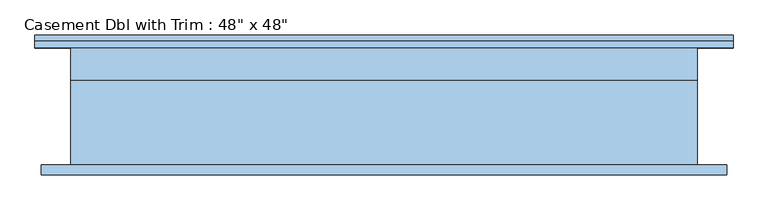
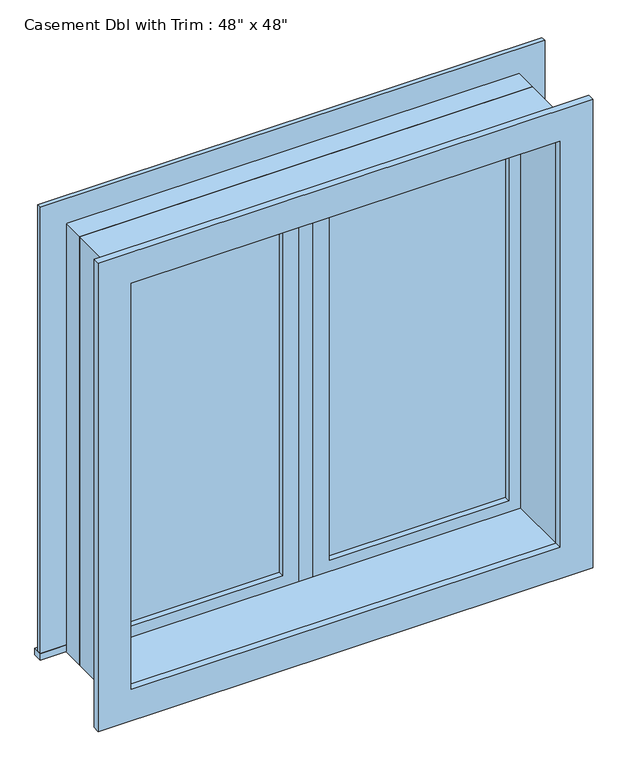
"""IFC4 building model written with IfcOpenShell, lengths in millimetres: window geometry."""

from ifc_helpers import new_model, si_unit, frame, origin, place, context, project, spatial, polyline, outline, extrude, source, transform, mapped, element, save


def window_534dcd48(model_context):
    return source(origin(), model_context, "Body", "SweptSolid", [
        extrude(outline(polyline([(63.5, 98.425), (546.1, 98.425), (546.1, 85.725), (63.5, 85.725), (63.5, 98.425)])), frame((0.0, 0.0, 977.9), z_axis=(0.0, 0.0, 1.0), x_axis=(1.0, 0.0, 0.0)), (0.0, 0.0, 1.0), 1092.2),
        extrude(outline(polyline([(2114.55, 19.05), (933.45, 19.05), (933.45, 590.55), (2114.55, 590.55), (2114.55, 19.05)]), holes=[polyline([(2070.1, 63.5), (2070.1, 546.1), (977.9, 546.1), (977.9, 63.5), (2070.1, 63.5)])]), frame((0.0, 69.85, 0.0), z_axis=(0.0, 1.0, 0.0), x_axis=(0.0, 0.0, 1.0)), (0.0, 0.0, 1.0), 44.45),
        extrude(outline(polyline([(19.05, 69.85), (-19.05, 69.85), (-19.05, 133.35), (19.05, 133.35), (19.05, 69.85)])), frame((0.0, 0.0, 933.45), z_axis=(0.0, 0.0, 1.0), x_axis=(1.0, 0.0, 0.0)), (0.0, 0.0, 1.0), 1181.1),
        extrude(outline(polyline([(-679.45, 158.75), (679.45, 158.75), (679.45, 133.35), (-679.45, 133.35), (-679.45, 158.75)])), frame((0.0, 0.0, 914.4), z_axis=(0.0, 0.0, 1.0), x_axis=(1.0, 0.0, 0.0)), (0.0, 0.0, 1.0), 19.05),
        extrude(outline(polyline([(2114.55, -590.55), (2114.55, 590.55), (933.45, 590.55), (933.45, 679.45), (2203.45, 679.45), (2203.45, -679.45), (933.45, -679.45), (933.45, -590.55), (2114.55, -590.55)])), frame((0.0, 133.35, 0.0), z_axis=(0.0, 1.0, 0.0), x_axis=(0.0, 0.0, 1.0)), (0.0, 0.0, 1.0), 12.7),
        extrude(outline(polyline([(2190.75, 666.75), (2190.75, -666.75), (857.25, -666.75), (857.25, 666.75), (2190.75, 666.75)]), holes=[polyline([(2101.85, 577.85), (946.15, 577.85), (946.15, -577.85), (2101.85, -577.85), (2101.85, 577.85)])]), frame((0.0, -114.3, 0.0), z_axis=(0.0, 1.0, 0.0), x_axis=(0.0, 0.0, 1.0)), (0.0, 0.0, 1.0), 19.05),
        extrude(outline(polyline([(-63.5, 85.725), (-546.1, 85.725), (-546.1, 98.425), (-63.5, 98.425), (-63.5, 85.725)])), frame((0.0, 0.0, 977.9), z_axis=(0.0, 0.0, 1.0), x_axis=(1.0, 0.0, 0.0)), (0.0, 0.0, 1.0), 1092.2),
        extrude(outline(polyline([(2114.55, -590.55), (933.45, -590.55), (933.45, -19.05), (2114.55, -19.05), (2114.55, -590.55)]), holes=[polyline([(2070.1, -546.1), (2070.1, -63.5), (977.9, -63.5), (977.9, -546.1), (2070.1, -546.1)])]), frame((0.0, 69.85, 0.0), z_axis=(0.0, 1.0, 0.0), x_axis=(0.0, 0.0, 1.0)), (0.0, 0.0, 1.0), 44.45),
        extrude(outline(polyline([(2133.6, -609.6), (914.4, -609.6), (914.4, 609.6), (2133.6, 609.6), (2133.6, -609.6)]), holes=[polyline([(2101.85, -577.85), (2101.85, 577.85), (946.15, 577.85), (946.15, -577.85), (2101.85, -577.85)])]), frame((0.0, -95.25, 0.0), z_axis=(0.0, 1.0, 0.0), x_axis=(0.0, 0.0, 1.0)), (0.0, 0.0, 1.0), 165.1),
        extrude(outline(polyline([(2133.6, 609.6), (2133.6, -609.6), (914.4, -609.6), (914.4, 609.6), (2133.6, 609.6)]), holes=[polyline([(2114.55, 590.55), (933.45, 590.55), (933.45, -590.55), (2114.55, -590.55), (2114.55, 590.55)])]), frame((0.0, 69.85, 0.0), z_axis=(0.0, 1.0, 0.0), x_axis=(0.0, 0.0, 1.0)), (0.0, 0.0, 1.0), 63.5),
    ])


if __name__ == "__main__":
    model = new_model("IFC4")
    model_context = context("Model", 3, world=origin())
    ifc_project = project(units=[si_unit("LENGTHUNIT", "METRE", prefix="MILLI")], contexts=[model_context])
    site = spatial("IfcSite", under=ifc_project)
    building = spatial("IfcBuilding", under=site)
    placement = place(None, origin())
    window_shape = window_534dcd48(model_context)
    element("IfcWindow", 1, ObjectType="Casement Dbl with Trim : 48\" x 48\"", at=placement, inside=building, context=model_context, shape_type="MappedRepresentation", body=[
        mapped(window_shape, transform((0.0, 0.0, 0.0), x_axis=(1.0, 0.0, 0.0), y_axis=(0.0, 1.0, 0.0), z_axis=(0.0, 0.0, 1.0))),
    ])
    save(model, "model.ifc")

# Revit data of these elements
# Type "Casement Dbl with Trim : 48\" x 48\""
#   Type Mark = "13"
#   Construction Type Id = "GSP4R"
#   Assembly Code = "B2020100"
#   Analytic Construction = "1/8 in Pilkington single glazing"
#   Visual Light Transmittance = 0.9
#   Solar Heat Gain Coefficient = 0.78
#   Heat Transfer Coefficient (U) = 0.6496 BTU/(h·ft²·°F)
#   Height = 4' - 0"
#   Default Sill Height = 3' - 0"
#   Trim Projection - Ext. = 0' - 0 1/2"
#   Trim Projection - Int. = 0' - 0 3/4"
#   Trim Width - Exterior = 0' - 3 1/2"
#   Trim Width - Interior = 0' - 3 1/2"
#   Width = 4' - 0"
#   Window Inset = 0' - 0 3/4"
#   Define Thermal Properties by = 1
#   Glass Pane Material = Glass
#   Sash Material = Sash
#   Trim Exterior Material = Trim
#   Trim Interior Material = Trim
#   Wall Closure = (empty or 0)
# Element 1 (IfcWindow, "Casement Dbl with Trim : 48\" x 48\"")
#   Materials on its faces: "Sash", "Trim", "Glass"
# Materials
#   "Glass": class "Glass", colour RGB 0 128 192, transparency 0.75, Description = "Soda Lime Glass", Cost = 0
#   "Sash": class "Wood", colour RGB 224 178 126, transparency 0
#   "Trim": class "Wood", colour RGB 224 178 126, transparency 0
